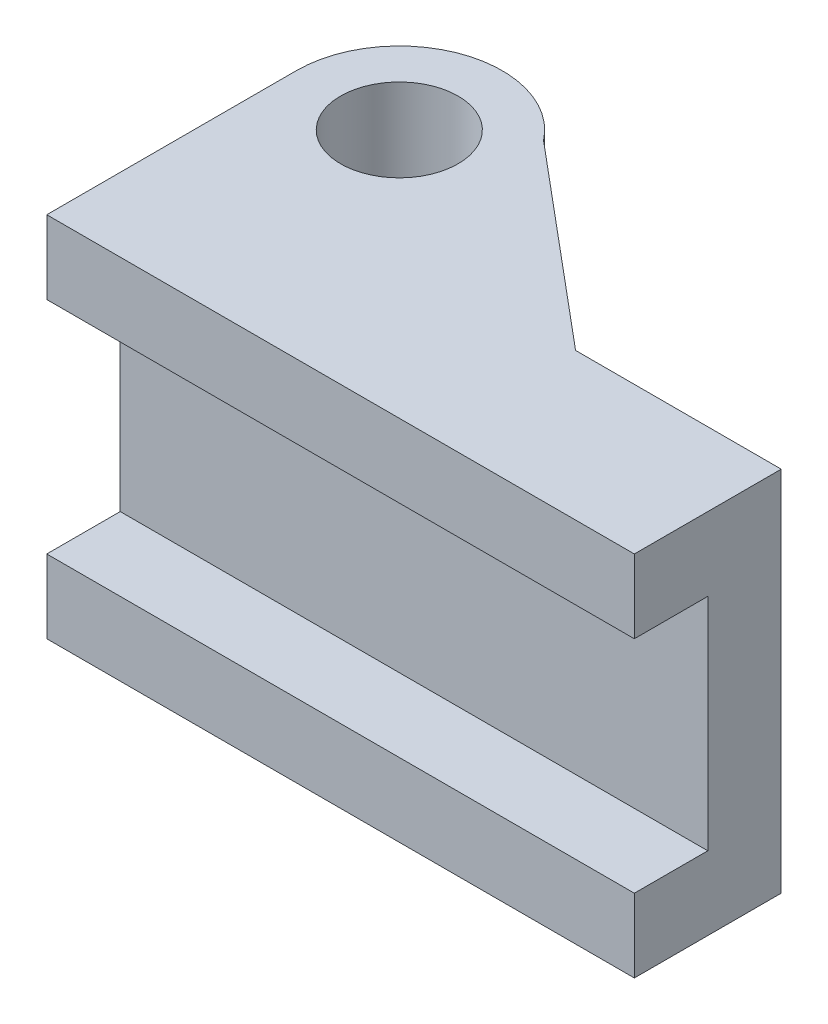
ISO-10303-21;
HEADER;
FILE_DESCRIPTION(('STEP AP214'),'2;1');
FILE_NAME('part.step','',(''),(''),'','','');
FILE_SCHEMA(('AUTOMOTIVE_DESIGN { 1 0 10303 214 1 1 1 1 }'));
ENDSEC;
DATA;
#1=APPLICATION_CONTEXT('core data for automotive mechanical design processes');
#2=APPLICATION_PROTOCOL_DEFINITION('international standard','automotive_design',2000,#1);
#3=PRODUCT_CONTEXT('',#1,'mechanical');
#4=PRODUCT('Part','Part','',(#3));
#5=PRODUCT_RELATED_PRODUCT_CATEGORY('part','',(#4));
#6=PRODUCT_DEFINITION_FORMATION('','',#4);
#7=PRODUCT_DEFINITION_CONTEXT('part definition',#1,'design');
#8=PRODUCT_DEFINITION('design','',#6,#7);
#9=PRODUCT_DEFINITION_SHAPE('','',#8);
#10=(LENGTH_UNIT() NAMED_UNIT(*) SI_UNIT(.MILLI.,.METRE.));
#11=(NAMED_UNIT(*) PLANE_ANGLE_UNIT() SI_UNIT($,.RADIAN.));
#12=(NAMED_UNIT(*) SI_UNIT($,.STERADIAN.) SOLID_ANGLE_UNIT());
#13=UNCERTAINTY_MEASURE_WITH_UNIT(LENGTH_MEASURE(1.E-05),#10,'distance_accuracy_value','');
#14=(GEOMETRIC_REPRESENTATION_CONTEXT(3) GLOBAL_UNCERTAINTY_ASSIGNED_CONTEXT((#13)) GLOBAL_UNIT_ASSIGNED_CONTEXT((#10,
#11,#12)) REPRESENTATION_CONTEXT('',''));
#15=CARTESIAN_POINT('',(0.,0.,0.));
#16=DIRECTION('',(0.,0.,1.));
#17=DIRECTION('',(1.,0.,0.));
#18=AXIS2_PLACEMENT_3D('',#15,#16,#17);
#19=CARTESIAN_POINT('',(0.,-125.,50.));
#20=DIRECTION('',(0.,0.939692620785908,0.342020143325669));
#21=DIRECTION('',(0.,-0.342020143325669,0.939692620785908));
#22=AXIS2_PLACEMENT_3D('',#19,#20,#21);
#23=PLANE('',#22);
#24=DIRECTION('',(0.,0.342020143325669,-0.939692620785908));
#25=VECTOR('',#24,1.);
#26=CARTESIAN_POINT('',(80.,-106.80148828669,0.));
#27=LINE('',#26,#25);
#28=CARTESIAN_POINT('',(80.,-125.,50.));
#29=VERTEX_POINT('',#28);
#30=CARTESIAN_POINT('',(80.,-106.80148828669,0.));
#31=VERTEX_POINT('',#30);
#32=EDGE_CURVE('E173',#29,#31,#27,.T.);
#33=ORIENTED_EDGE('',*,*,#32,.T.);
#34=DIRECTION('',(-1.,0.,0.));
#35=VECTOR('',#34,1.);
#36=CARTESIAN_POINT('',(0.,-106.80148828669,0.));
#37=LINE('',#36,#35);
#38=CARTESIAN_POINT('',(120.,-106.80148828669,0.));
#39=VERTEX_POINT('',#38);
#40=EDGE_CURVE('E11',#39,#31,#37,.T.);
#41=ORIENTED_EDGE('',*,*,#40,.F.);
#42=DIRECTION('',(0.,-0.342020143325669,0.939692620785908));
#43=VECTOR('',#42,1.);
#44=CARTESIAN_POINT('',(120.,-125.,50.));
#45=LINE('',#44,#43);
#46=CARTESIAN_POINT('',(120.,-125.,50.));
#47=VERTEX_POINT('',#46);
#48=EDGE_CURVE('E194',#39,#47,#45,.T.);
#49=ORIENTED_EDGE('',*,*,#48,.T.);
#50=DIRECTION('',(1.,0.,0.));
#51=VECTOR('',#50,1.);
#52=CARTESIAN_POINT('',(0.,-125.,50.));
#53=LINE('',#52,#51);
#54=EDGE_CURVE('E61',#29,#47,#53,.T.);
#55=ORIENTED_EDGE('',*,*,#54,.F.);
#56=EDGE_LOOP('',(#33,#41,#49,#55));
#57=FACE_BOUND('',#56,.T.);
#58=ADVANCED_FACE('F50',(#57),#23,.F.);
#59=CARTESIAN_POINT('',(0.,0.,50.));
#60=DIRECTION('',(0.,0.,1.));
#61=DIRECTION('',(1.,0.,0.));
#62=AXIS2_PLACEMENT_3D('',#59,#60,#61);
#63=PLANE('',#62);
#64=DIRECTION('',(1.,0.,0.));
#65=VECTOR('',#64,1.);
#66=CARTESIAN_POINT('',(0.,-25.,50.));
#67=LINE('',#66,#65);
#68=CARTESIAN_POINT('',(0.,-25.,50.));
#69=VERTEX_POINT('',#68);
#70=CARTESIAN_POINT('',(200.,-25.,50.));
#71=VERTEX_POINT('',#70);
#72=EDGE_CURVE('E220',#69,#71,#67,.T.);
#73=ORIENTED_EDGE('',*,*,#72,.T.);
#74=DIRECTION('',(0.,1.,0.));
#75=VECTOR('',#74,1.);
#76=CARTESIAN_POINT('',(200.,-125.,50.));
#77=LINE('',#76,#75);
#78=CARTESIAN_POINT('',(200.,0.,50.));
#79=VERTEX_POINT('',#78);
#80=EDGE_CURVE('E285',#71,#79,#77,.T.);
#81=ORIENTED_EDGE('',*,*,#80,.T.);
#82=DIRECTION('',(-1.,0.,0.));
#83=VECTOR('',#82,1.);
#84=CARTESIAN_POINT('',(200.,0.,50.));
#85=LINE('',#84,#83);
#86=CARTESIAN_POINT('',(0.,0.,50.));
#87=VERTEX_POINT('',#86);
#88=EDGE_CURVE('E275',#79,#87,#85,.T.);
#89=ORIENTED_EDGE('',*,*,#88,.T.);
#90=DIRECTION('',(0.,-1.,0.));
#91=VECTOR('',#90,1.);
#92=CARTESIAN_POINT('',(0.,0.,50.));
#93=LINE('',#92,#91);
#94=EDGE_CURVE('E276',#87,#69,#93,.T.);
#95=ORIENTED_EDGE('',*,*,#94,.T.);
#96=EDGE_LOOP('',(#73,#81,#89,#95));
#97=FACE_BOUND('',#96,.T.);
#98=ADVANCED_FACE('F347',(#97),#63,.T.);
#99=CARTESIAN_POINT('',(70.,-50.,0.));
#100=DIRECTION('',(1.,0.,0.));
#101=DIRECTION('',(0.,0.,-1.));
#102=AXIS2_PLACEMENT_3D('',#99,#100,#101);
#103=PLANE('',#102);
#104=DIRECTION('',(0.,1.,0.));
#105=VECTOR('',#104,1.);
#106=CARTESIAN_POINT('',(70.,-50.,-35.));
#107=LINE('',#106,#105);
#108=CARTESIAN_POINT('',(70.,-50.,-35.));
#109=VERTEX_POINT('',#108);
#110=CARTESIAN_POINT('',(70.,-30.,-35.));
#111=VERTEX_POINT('',#110);
#112=EDGE_CURVE('E270',#109,#111,#107,.T.);
#113=ORIENTED_EDGE('',*,*,#112,.T.);
#114=DIRECTION('',(0.,0.,-1.));
#115=VECTOR('',#114,1.);
#116=CARTESIAN_POINT('',(70.,-30.,0.));
#117=LINE('',#116,#115);
#118=CARTESIAN_POINT('',(70.,-30.,0.));
#119=VERTEX_POINT('',#118);
#120=EDGE_CURVE('E237',#119,#111,#117,.T.);
#121=ORIENTED_EDGE('',*,*,#120,.F.);
#122=DIRECTION('',(0.,1.,0.));
#123=VECTOR('',#122,1.);
#124=CARTESIAN_POINT('',(70.,-50.,0.));
#125=LINE('',#124,#123);
#126=CARTESIAN_POINT('',(70.,-50.,0.));
#127=VERTEX_POINT('',#126);
#128=EDGE_CURVE('E261',#127,#119,#125,.T.);
#129=ORIENTED_EDGE('',*,*,#128,.F.);
#130=DIRECTION('',(0.,0.,-1.));
#131=VECTOR('',#130,1.);
#132=CARTESIAN_POINT('',(70.,-50.,0.));
#133=LINE('',#132,#131);
#134=EDGE_CURVE('E253',#127,#109,#133,.T.);
#135=ORIENTED_EDGE('',*,*,#134,.T.);
#136=EDGE_LOOP('',(#113,#121,#129,#135));
#137=FACE_BOUND('',#136,.T.);
#138=ADVANCED_FACE('F315',(#137),#103,.T.);
#139=CARTESIAN_POINT('',(200.,0.,50.));
#140=DIRECTION('',(0.,-1.,0.));
#141=DIRECTION('',(0.,0.,-1.));
#142=AXIS2_PLACEMENT_3D('',#139,#140,#141);
#143=PLANE('',#142);
#144=CARTESIAN_POINT('',(35.,0.,-35.));
#145=DIRECTION('',(0.,-1.,0.));
#146=DIRECTION('',(0.,0.,-1.));
#147=AXIS2_PLACEMENT_3D('',#144,#145,#146);
#148=CIRCLE('',#147,20.);
#149=CARTESIAN_POINT('',(35.,0.,-55.));
#150=VERTEX_POINT('',#149);
#151=EDGE_CURVE('E228',#150,#150,#148,.T.);
#152=ORIENTED_EDGE('',*,*,#151,.T.);
#153=EDGE_LOOP('',(#152));
#154=FACE_BOUND('',#153,.T.);
#155=DIRECTION('',(-0.766441896118766,0.,-0.642313646028068));
#156=VECTOR('',#155,1.);
#157=CARTESIAN_POINT('',(53.6336865836032,0.,-63.9984915394124));
#158=LINE('',#157,#156);
#159=CARTESIAN_POINT('',(130.,0.,0.));
#160=VERTEX_POINT('',#159);
#161=CARTESIAN_POINT('',(62.6860807533592,0.,-56.4121678612529));
#162=VERTEX_POINT('',#161);
#163=EDGE_CURVE('E230',#160,#162,#158,.T.);
#164=ORIENTED_EDGE('',*,*,#163,.T.);
#165=CARTESIAN_POINT('',(35.,0.,-35.));
#166=DIRECTION('',(0.,1.,0.));
#167=DIRECTION('',(0.,0.,1.));
#168=AXIS2_PLACEMENT_3D('',#165,#166,#167);
#169=CIRCLE('',#168,35.);
#170=CARTESIAN_POINT('',(0.,0.,-35.));
#171=VERTEX_POINT('',#170);
#172=EDGE_CURVE('E246',#162,#171,#169,.T.);
#173=ORIENTED_EDGE('',*,*,#172,.T.);
#174=DIRECTION('',(0.,0.,-1.));
#175=VECTOR('',#174,1.);
#176=CARTESIAN_POINT('',(0.,0.,50.));
#177=LINE('',#176,#175);
#178=EDGE_CURVE('E54',#87,#171,#177,.T.);
#179=ORIENTED_EDGE('',*,*,#178,.F.);
#180=ORIENTED_EDGE('',*,*,#88,.F.);
#181=DIRECTION('',(0.,0.,-1.));
#182=VECTOR('',#181,1.);
#183=CARTESIAN_POINT('',(200.,0.,50.));
#184=LINE('',#183,#182);
#185=CARTESIAN_POINT('',(200.,0.,0.));
#186=VERTEX_POINT('',#185);
#187=EDGE_CURVE('E288',#79,#186,#184,.T.);
#188=ORIENTED_EDGE('',*,*,#187,.T.);
#189=DIRECTION('',(-1.,0.,0.));
#190=VECTOR('',#189,1.);
#191=CARTESIAN_POINT('',(200.,0.,0.));
#192=LINE('',#191,#190);
#193=EDGE_CURVE('E268',#186,#160,#192,.T.);
#194=ORIENTED_EDGE('',*,*,#193,.T.);
#195=EDGE_LOOP('',(#164,#173,#179,#180,#188,#194));
#196=FACE_BOUND('',#195,.T.);
#197=ADVANCED_FACE('F47',(#154,#196),#143,.F.);
#198=CARTESIAN_POINT('',(0.,0.,50.));
#199=DIRECTION('',(1.,0.,0.));
#200=DIRECTION('',(0.,0.,-1.));
#201=AXIS2_PLACEMENT_3D('',#198,#199,#200);
#202=PLANE('',#201);
#203=DIRECTION('',(0.,-1.,0.));
#204=VECTOR('',#203,1.);
#205=CARTESIAN_POINT('',(0.,0.,0.));
#206=LINE('',#205,#204);
#207=CARTESIAN_POINT('',(0.,-50.,0.));
#208=VERTEX_POINT('',#207);
#209=CARTESIAN_POINT('',(0.,-125.,0.));
#210=VERTEX_POINT('',#209);
#211=EDGE_CURVE('E287',#208,#210,#206,.T.);
#212=ORIENTED_EDGE('',*,*,#211,.T.);
#213=DIRECTION('',(0.,0.,1.));
#214=VECTOR('',#213,1.);
#215=CARTESIAN_POINT('',(0.,-125.,50.));
#216=LINE('',#215,#214);
#217=CARTESIAN_POINT('',(0.,-125.,50.));
#218=VERTEX_POINT('',#217);
#219=EDGE_CURVE('E166',#210,#218,#216,.T.);
#220=ORIENTED_EDGE('',*,*,#219,.T.);
#221=CARTESIAN_POINT('',(0.,-100.,50.));
#222=VERTEX_POINT('',#221);
#223=EDGE_CURVE('E273',#222,#218,#93,.T.);
#224=ORIENTED_EDGE('',*,*,#223,.F.);
#225=DIRECTION('',(0.,0.,-1.));
#226=VECTOR('',#225,1.);
#227=CARTESIAN_POINT('',(0.,-100.,25.));
#228=LINE('',#227,#226);
#229=CARTESIAN_POINT('',(0.,-100.,25.));
#230=VERTEX_POINT('',#229);
#231=EDGE_CURVE('E69',#222,#230,#228,.T.);
#232=ORIENTED_EDGE('',*,*,#231,.T.);
#233=DIRECTION('',(0.,1.,0.));
#234=VECTOR('',#233,1.);
#235=CARTESIAN_POINT('',(0.,-25.,25.));
#236=LINE('',#235,#234);
#237=CARTESIAN_POINT('',(0.,-25.,25.));
#238=VERTEX_POINT('',#237);
#239=EDGE_CURVE('E201',#230,#238,#236,.T.);
#240=ORIENTED_EDGE('',*,*,#239,.T.);
#241=DIRECTION('',(0.,0.,1.));
#242=VECTOR('',#241,1.);
#243=CARTESIAN_POINT('',(0.,-25.,50.));
#244=LINE('',#243,#242);
#245=EDGE_CURVE('E210',#238,#69,#244,.T.);
#246=ORIENTED_EDGE('',*,*,#245,.T.);
#247=ORIENTED_EDGE('',*,*,#94,.F.);
#248=ORIENTED_EDGE('',*,*,#178,.T.);
#249=DIRECTION('',(0.,1.,0.));
#250=VECTOR('',#249,1.);
#251=CARTESIAN_POINT('',(0.,-50.,-35.));
#252=LINE('',#251,#250);
#253=CARTESIAN_POINT('',(0.,-50.,-35.));
#254=VERTEX_POINT('',#253);
#255=EDGE_CURVE('E262',#254,#171,#252,.T.);
#256=ORIENTED_EDGE('',*,*,#255,.F.);
#257=DIRECTION('',(0.,0.,1.));
#258=VECTOR('',#257,1.);
#259=CARTESIAN_POINT('',(0.,-50.,-35.));
#260=LINE('',#259,#258);
#261=EDGE_CURVE('E248',#254,#208,#260,.T.);
#262=ORIENTED_EDGE('',*,*,#261,.T.);
#263=EDGE_LOOP('',(#212,#220,#224,#232,#240,#246,#247,#248,#256,#262));
#264=FACE_BOUND('',#263,.T.);
#265=ADVANCED_FACE('F298',(#264),#202,.F.);
#266=CARTESIAN_POINT('',(200.,-125.,50.));
#267=DIRECTION('',(-1.,0.,0.));
#268=DIRECTION('',(0.,0.,1.));
#269=AXIS2_PLACEMENT_3D('',#266,#267,#268);
#270=PLANE('',#269);
#271=CARTESIAN_POINT('',(200.,-125.,50.));
#272=VERTEX_POINT('',#271);
#273=CARTESIAN_POINT('',(200.,-100.,50.));
#274=VERTEX_POINT('',#273);
#275=EDGE_CURVE('E282',#272,#274,#77,.T.);
#276=ORIENTED_EDGE('',*,*,#275,.F.);
#277=DIRECTION('',(0.,0.,-1.));
#278=VECTOR('',#277,1.);
#279=CARTESIAN_POINT('',(200.,-125.,0.));
#280=LINE('',#279,#278);
#281=CARTESIAN_POINT('',(200.,-125.,0.));
#282=VERTEX_POINT('',#281);
#283=EDGE_CURVE('E175',#272,#282,#280,.T.);
#284=ORIENTED_EDGE('',*,*,#283,.T.);
#285=DIRECTION('',(0.,1.,0.));
#286=VECTOR('',#285,1.);
#287=CARTESIAN_POINT('',(200.,-125.,0.));
#288=LINE('',#287,#286);
#289=EDGE_CURVE('E279',#282,#186,#288,.T.);
#290=ORIENTED_EDGE('',*,*,#289,.T.);
#291=ORIENTED_EDGE('',*,*,#187,.F.);
#292=ORIENTED_EDGE('',*,*,#80,.F.);
#293=DIRECTION('',(0.,0.,1.));
#294=VECTOR('',#293,1.);
#295=CARTESIAN_POINT('',(200.,-25.,50.));
#296=LINE('',#295,#294);
#297=CARTESIAN_POINT('',(200.,-25.,25.));
#298=VERTEX_POINT('',#297);
#299=EDGE_CURVE('E202',#298,#71,#296,.T.);
#300=ORIENTED_EDGE('',*,*,#299,.F.);
#301=DIRECTION('',(0.,1.,0.));
#302=VECTOR('',#301,1.);
#303=CARTESIAN_POINT('',(200.,-25.,25.));
#304=LINE('',#303,#302);
#305=CARTESIAN_POINT('',(200.,-100.,25.));
#306=VERTEX_POINT('',#305);
#307=EDGE_CURVE('E215',#306,#298,#304,.T.);
#308=ORIENTED_EDGE('',*,*,#307,.F.);
#309=DIRECTION('',(0.,0.,-1.));
#310=VECTOR('',#309,1.);
#311=CARTESIAN_POINT('',(200.,-100.,25.));
#312=LINE('',#311,#310);
#313=EDGE_CURVE('E198',#274,#306,#312,.T.);
#314=ORIENTED_EDGE('',*,*,#313,.F.);
#315=EDGE_LOOP('',(#276,#284,#290,#291,#292,#300,#308,#314));
#316=FACE_BOUND('',#315,.T.);
#317=ADVANCED_FACE('F326',(#316),#270,.F.);
#318=DIRECTION('',(1.,0.,0.));
#319=VECTOR('',#318,1.);
#320=CARTESIAN_POINT('',(0.,-100.,50.));
#321=LINE('',#320,#319);
#322=EDGE_CURVE('E208',#222,#274,#321,.T.);
#323=ORIENTED_EDGE('',*,*,#322,.F.);
#324=ORIENTED_EDGE('',*,*,#223,.T.);
#325=EDGE_CURVE('E277',#218,#29,#53,.T.);
#326=ORIENTED_EDGE('',*,*,#325,.T.);
#327=ORIENTED_EDGE('',*,*,#54,.T.);
#328=DIRECTION('',(1.,0.,0.));
#329=VECTOR('',#328,1.);
#330=CARTESIAN_POINT('',(120.,-125.,50.));
#331=LINE('',#330,#329);
#332=EDGE_CURVE('E200',#47,#272,#331,.T.);
#333=ORIENTED_EDGE('',*,*,#332,.T.);
#334=ORIENTED_EDGE('',*,*,#275,.T.);
#335=EDGE_LOOP('',(#323,#324,#326,#327,#333,#334));
#336=FACE_BOUND('',#335,.T.);
#337=ADVANCED_FACE('F328',(#336),#63,.T.);
#338=CARTESIAN_POINT('',(0.,0.,0.));
#339=DIRECTION('',(0.,0.,1.));
#340=DIRECTION('',(1.,0.,0.));
#341=AXIS2_PLACEMENT_3D('',#338,#339,#340);
#342=PLANE('',#341);
#343=ORIENTED_EDGE('',*,*,#289,.F.);
#344=DIRECTION('',(1.,0.,0.));
#345=VECTOR('',#344,1.);
#346=CARTESIAN_POINT('',(120.,-125.,0.));
#347=LINE('',#346,#345);
#348=CARTESIAN_POINT('',(120.,-125.,0.));
#349=VERTEX_POINT('',#348);
#350=EDGE_CURVE('E193',#349,#282,#347,.T.);
#351=ORIENTED_EDGE('',*,*,#350,.F.);
#352=DIRECTION('',(0.,1.,0.));
#353=VECTOR('',#352,1.);
#354=CARTESIAN_POINT('',(120.,-106.80148828669,0.));
#355=LINE('',#354,#353);
#356=EDGE_CURVE('E186',#349,#39,#355,.T.);
#357=ORIENTED_EDGE('',*,*,#356,.T.);
#358=ORIENTED_EDGE('',*,*,#40,.T.);
#359=DIRECTION('',(0.,-1.,0.));
#360=VECTOR('',#359,1.);
#361=CARTESIAN_POINT('',(80.,-125.,0.));
#362=LINE('',#361,#360);
#363=CARTESIAN_POINT('',(80.,-125.,0.));
#364=VERTEX_POINT('',#363);
#365=EDGE_CURVE('E180',#31,#364,#362,.T.);
#366=ORIENTED_EDGE('',*,*,#365,.T.);
#367=DIRECTION('',(-1.,0.,0.));
#368=VECTOR('',#367,1.);
#369=CARTESIAN_POINT('',(80.,-125.,0.));
#370=LINE('',#369,#368);
#371=EDGE_CURVE('E162',#364,#210,#370,.T.);
#372=ORIENTED_EDGE('',*,*,#371,.T.);
#373=ORIENTED_EDGE('',*,*,#211,.F.);
#374=DIRECTION('',(1.,0.,0.));
#375=VECTOR('',#374,1.);
#376=CARTESIAN_POINT('',(0.,-50.,0.));
#377=LINE('',#376,#375);
#378=EDGE_CURVE('E255',#208,#127,#377,.T.);
#379=ORIENTED_EDGE('',*,*,#378,.T.);
#380=ORIENTED_EDGE('',*,*,#128,.T.);
#381=DIRECTION('',(-1.,0.,0.));
#382=VECTOR('',#381,1.);
#383=CARTESIAN_POINT('',(0.,-30.,0.));
#384=LINE('',#383,#382);
#385=CARTESIAN_POINT('',(130.,-30.,0.));
#386=VERTEX_POINT('',#385);
#387=EDGE_CURVE('E235',#386,#119,#384,.T.);
#388=ORIENTED_EDGE('',*,*,#387,.F.);
#389=DIRECTION('',(0.,1.,0.));
#390=VECTOR('',#389,1.);
#391=CARTESIAN_POINT('',(130.,-30.,0.));
#392=LINE('',#391,#390);
#393=EDGE_CURVE('E241',#386,#160,#392,.T.);
#394=ORIENTED_EDGE('',*,*,#393,.T.);
#395=ORIENTED_EDGE('',*,*,#193,.F.);
#396=EDGE_LOOP('',(#343,#351,#357,#358,#366,#372,#373,#379,#380,#388,#394,#395));
#397=FACE_BOUND('',#396,.T.);
#398=ADVANCED_FACE('F179',(#397),#342,.F.);
#399=CARTESIAN_POINT('',(35.,-50.,-35.));
#400=DIRECTION('',(0.,1.,0.));
#401=DIRECTION('',(0.,0.,1.));
#402=AXIS2_PLACEMENT_3D('',#399,#400,#401);
#403=CYLINDRICAL_SURFACE('',#402,35.);
#404=DIRECTION('',(0.,1.,0.));
#405=VECTOR('',#404,1.);
#406=CARTESIAN_POINT('',(62.6860807533592,-30.,-56.4121678612529));
#407=LINE('',#406,#405);
#408=CARTESIAN_POINT('',(62.6860807533592,-30.,-56.4121678612529));
#409=VERTEX_POINT('',#408);
#410=EDGE_CURVE('E242',#409,#162,#407,.T.);
#411=ORIENTED_EDGE('',*,*,#410,.F.);
#412=CARTESIAN_POINT('',(35.,-30.,-35.));
#413=DIRECTION('',(0.,1.,0.));
#414=DIRECTION('',(0.,0.,1.));
#415=AXIS2_PLACEMENT_3D('',#412,#413,#414);
#416=CIRCLE('',#415,35.);
#417=EDGE_CURVE('E240',#111,#409,#416,.T.);
#418=ORIENTED_EDGE('',*,*,#417,.F.);
#419=ORIENTED_EDGE('',*,*,#112,.F.);
#420=CARTESIAN_POINT('',(35.,-50.,-35.));
#421=DIRECTION('',(0.,1.,0.));
#422=DIRECTION('',(0.,0.,1.));
#423=AXIS2_PLACEMENT_3D('',#420,#421,#422);
#424=CIRCLE('',#423,35.);
#425=EDGE_CURVE('E260',#109,#254,#424,.T.);
#426=ORIENTED_EDGE('',*,*,#425,.T.);
#427=ORIENTED_EDGE('',*,*,#255,.T.);
#428=ORIENTED_EDGE('',*,*,#172,.F.);
#429=EDGE_LOOP('',(#411,#418,#419,#426,#427,#428));
#430=FACE_BOUND('',#429,.T.);
#431=ADVANCED_FACE('F303',(#430),#403,.T.);
#432=CARTESIAN_POINT('',(35.,-50.,-35.));
#433=DIRECTION('',(0.,1.,0.));
#434=DIRECTION('',(0.,0.,1.));
#435=AXIS2_PLACEMENT_3D('',#432,#433,#434);
#436=PLANE('',#435);
#437=CARTESIAN_POINT('',(35.,-50.,-35.));
#438=DIRECTION('',(0.,-1.,0.));
#439=DIRECTION('',(0.,0.,-1.));
#440=AXIS2_PLACEMENT_3D('',#437,#438,#439);
#441=CIRCLE('',#440,20.);
#442=CARTESIAN_POINT('',(35.,-50.,-55.));
#443=VERTEX_POINT('',#442);
#444=EDGE_CURVE('E219',#443,#443,#441,.T.);
#445=ORIENTED_EDGE('',*,*,#444,.F.);
#446=EDGE_LOOP('',(#445));
#447=FACE_BOUND('',#446,.T.);
#448=ORIENTED_EDGE('',*,*,#261,.F.);
#449=ORIENTED_EDGE('',*,*,#425,.F.);
#450=ORIENTED_EDGE('',*,*,#134,.F.);
#451=ORIENTED_EDGE('',*,*,#378,.F.);
#452=EDGE_LOOP('',(#448,#449,#450,#451));
#453=FACE_BOUND('',#452,.T.);
#454=ADVANCED_FACE('F308',(#447,#453),#436,.F.);
#455=CARTESIAN_POINT('',(53.6336865836032,-30.,-63.9984915394124));
#456=DIRECTION('',(0.642313646028068,0.,-0.766441896118766));
#457=DIRECTION('',(-0.766441896118766,0.,-0.642313646028068));
#458=AXIS2_PLACEMENT_3D('',#455,#456,#457);
#459=PLANE('',#458);
#460=ORIENTED_EDGE('',*,*,#163,.F.);
#461=ORIENTED_EDGE('',*,*,#393,.F.);
#462=DIRECTION('',(-0.766441896118766,0.,-0.642313646028068));
#463=VECTOR('',#462,1.);
#464=CARTESIAN_POINT('',(53.6336865836032,-30.,-63.9984915394124));
#465=LINE('',#464,#463);
#466=EDGE_CURVE('E234',#386,#409,#465,.T.);
#467=ORIENTED_EDGE('',*,*,#466,.T.);
#468=ORIENTED_EDGE('',*,*,#410,.T.);
#469=EDGE_LOOP('',(#460,#461,#467,#468));
#470=FACE_BOUND('',#469,.T.);
#471=ADVANCED_FACE('F320',(#470),#459,.T.);
#472=CARTESIAN_POINT('',(0.,-30.,0.));
#473=DIRECTION('',(0.,1.,0.));
#474=DIRECTION('',(0.,0.,1.));
#475=AXIS2_PLACEMENT_3D('',#472,#473,#474);
#476=PLANE('',#475);
#477=ORIENTED_EDGE('',*,*,#387,.T.);
#478=ORIENTED_EDGE('',*,*,#120,.T.);
#479=ORIENTED_EDGE('',*,*,#417,.T.);
#480=ORIENTED_EDGE('',*,*,#466,.F.);
#481=EDGE_LOOP('',(#477,#478,#479,#480));
#482=FACE_BOUND('',#481,.T.);
#483=ADVANCED_FACE('F313',(#482),#476,.F.);
#484=CARTESIAN_POINT('',(35.,0.,-35.));
#485=DIRECTION('',(0.,-1.,0.));
#486=DIRECTION('',(0.,0.,-1.));
#487=AXIS2_PLACEMENT_3D('',#484,#485,#486);
#488=CYLINDRICAL_SURFACE('',#487,20.);
#489=ORIENTED_EDGE('',*,*,#151,.F.);
#490=EDGE_LOOP('',(#489));
#491=FACE_BOUND('',#490,.T.);
#492=ORIENTED_EDGE('',*,*,#444,.T.);
#493=EDGE_LOOP('',(#492));
#494=FACE_BOUND('',#493,.T.);
#495=ADVANCED_FACE('F363',(#491,#494),#488,.F.);
#496=CARTESIAN_POINT('',(0.,-25.,50.));
#497=DIRECTION('',(0.,1.,0.));
#498=DIRECTION('',(0.,0.,1.));
#499=AXIS2_PLACEMENT_3D('',#496,#497,#498);
#500=PLANE('',#499);
#501=ORIENTED_EDGE('',*,*,#299,.T.);
#502=ORIENTED_EDGE('',*,*,#72,.F.);
#503=ORIENTED_EDGE('',*,*,#245,.F.);
#504=DIRECTION('',(1.,0.,0.));
#505=VECTOR('',#504,1.);
#506=CARTESIAN_POINT('',(0.,-25.,25.));
#507=LINE('',#506,#505);
#508=EDGE_CURVE('E223',#238,#298,#507,.T.);
#509=ORIENTED_EDGE('',*,*,#508,.T.);
#510=EDGE_LOOP('',(#501,#502,#503,#509));
#511=FACE_BOUND('',#510,.T.);
#512=ADVANCED_FACE('F357',(#511),#500,.F.);
#513=CARTESIAN_POINT('',(0.,-25.,25.));
#514=DIRECTION('',(0.,0.,-1.));
#515=DIRECTION('',(-1.,0.,0.));
#516=AXIS2_PLACEMENT_3D('',#513,#514,#515);
#517=PLANE('',#516);
#518=ORIENTED_EDGE('',*,*,#307,.T.);
#519=ORIENTED_EDGE('',*,*,#508,.F.);
#520=ORIENTED_EDGE('',*,*,#239,.F.);
#521=DIRECTION('',(1.,0.,0.));
#522=VECTOR('',#521,1.);
#523=CARTESIAN_POINT('',(0.,-100.,25.));
#524=LINE('',#523,#522);
#525=EDGE_CURVE('E221',#230,#306,#524,.T.);
#526=ORIENTED_EDGE('',*,*,#525,.T.);
#527=EDGE_LOOP('',(#518,#519,#520,#526));
#528=FACE_BOUND('',#527,.T.);
#529=ADVANCED_FACE('F359',(#528),#517,.F.);
#530=CARTESIAN_POINT('',(0.,-100.,25.));
#531=DIRECTION('',(0.,-1.,0.));
#532=DIRECTION('',(0.,0.,-1.));
#533=AXIS2_PLACEMENT_3D('',#530,#531,#532);
#534=PLANE('',#533);
#535=ORIENTED_EDGE('',*,*,#313,.T.);
#536=ORIENTED_EDGE('',*,*,#525,.F.);
#537=ORIENTED_EDGE('',*,*,#231,.F.);
#538=ORIENTED_EDGE('',*,*,#322,.T.);
#539=EDGE_LOOP('',(#535,#536,#537,#538));
#540=FACE_BOUND('',#539,.T.);
#541=ADVANCED_FACE('F342',(#540),#534,.F.);
#542=CARTESIAN_POINT('',(120.,-125.,0.));
#543=DIRECTION('',(0.,-1.,0.));
#544=DIRECTION('',(0.,0.,-1.));
#545=AXIS2_PLACEMENT_3D('',#542,#543,#544);
#546=PLANE('',#545);
#547=ORIENTED_EDGE('',*,*,#283,.F.);
#548=ORIENTED_EDGE('',*,*,#332,.F.);
#549=DIRECTION('',(0.,0.,-1.));
#550=VECTOR('',#549,1.);
#551=CARTESIAN_POINT('',(120.,-125.,0.));
#552=LINE('',#551,#550);
#553=EDGE_CURVE('E187',#47,#349,#552,.T.);
#554=ORIENTED_EDGE('',*,*,#553,.T.);
#555=ORIENTED_EDGE('',*,*,#350,.T.);
#556=EDGE_LOOP('',(#547,#548,#554,#555));
#557=FACE_BOUND('',#556,.T.);
#558=ADVANCED_FACE('F325',(#557),#546,.T.);
#559=CARTESIAN_POINT('',(120.,0.,0.));
#560=DIRECTION('',(1.,0.,0.));
#561=DIRECTION('',(0.,0.,-1.));
#562=AXIS2_PLACEMENT_3D('',#559,#560,#561);
#563=PLANE('',#562);
#564=ORIENTED_EDGE('',*,*,#553,.F.);
#565=ORIENTED_EDGE('',*,*,#48,.F.);
#566=ORIENTED_EDGE('',*,*,#356,.F.);
#567=EDGE_LOOP('',(#564,#565,#566));
#568=FACE_BOUND('',#567,.T.);
#569=ADVANCED_FACE('F334',(#568),#563,.F.);
#570=CARTESIAN_POINT('',(80.,-125.,50.));
#571=DIRECTION('',(0.,-1.,0.));
#572=DIRECTION('',(0.,0.,-1.));
#573=AXIS2_PLACEMENT_3D('',#570,#571,#572);
#574=PLANE('',#573);
#575=ORIENTED_EDGE('',*,*,#219,.F.);
#576=ORIENTED_EDGE('',*,*,#371,.F.);
#577=DIRECTION('',(0.,0.,1.));
#578=VECTOR('',#577,1.);
#579=CARTESIAN_POINT('',(80.,-125.,50.));
#580=LINE('',#579,#578);
#581=EDGE_CURVE('E168',#364,#29,#580,.T.);
#582=ORIENTED_EDGE('',*,*,#581,.T.);
#583=ORIENTED_EDGE('',*,*,#325,.F.);
#584=EDGE_LOOP('',(#575,#576,#582,#583));
#585=FACE_BOUND('',#584,.T.);
#586=ADVANCED_FACE('F165',(#585),#574,.T.);
#587=CARTESIAN_POINT('',(80.,0.,0.));
#588=DIRECTION('',(-1.,0.,0.));
#589=DIRECTION('',(0.,0.,1.));
#590=AXIS2_PLACEMENT_3D('',#587,#588,#589);
#591=PLANE('',#590);
#592=ORIENTED_EDGE('',*,*,#365,.F.);
#593=ORIENTED_EDGE('',*,*,#32,.F.);
#594=ORIENTED_EDGE('',*,*,#581,.F.);
#595=EDGE_LOOP('',(#592,#593,#594));
#596=FACE_BOUND('',#595,.T.);
#597=ADVANCED_FACE('F176',(#596),#591,.F.);
#598=CLOSED_SHELL('',(#58,#98,#138,#197,#265,#317,#337,#398,#431,#454,#471,#483,#495,#512,#529,
#541,#558,#569,#586,#597));
#599=MANIFOLD_SOLID_BREP('B2',#598);
#600=ADVANCED_BREP_SHAPE_REPRESENTATION('',(#18,#599),#14);
#601=SHAPE_DEFINITION_REPRESENTATION(#9,#600);
ENDSEC;
END-ISO-10303-21;
